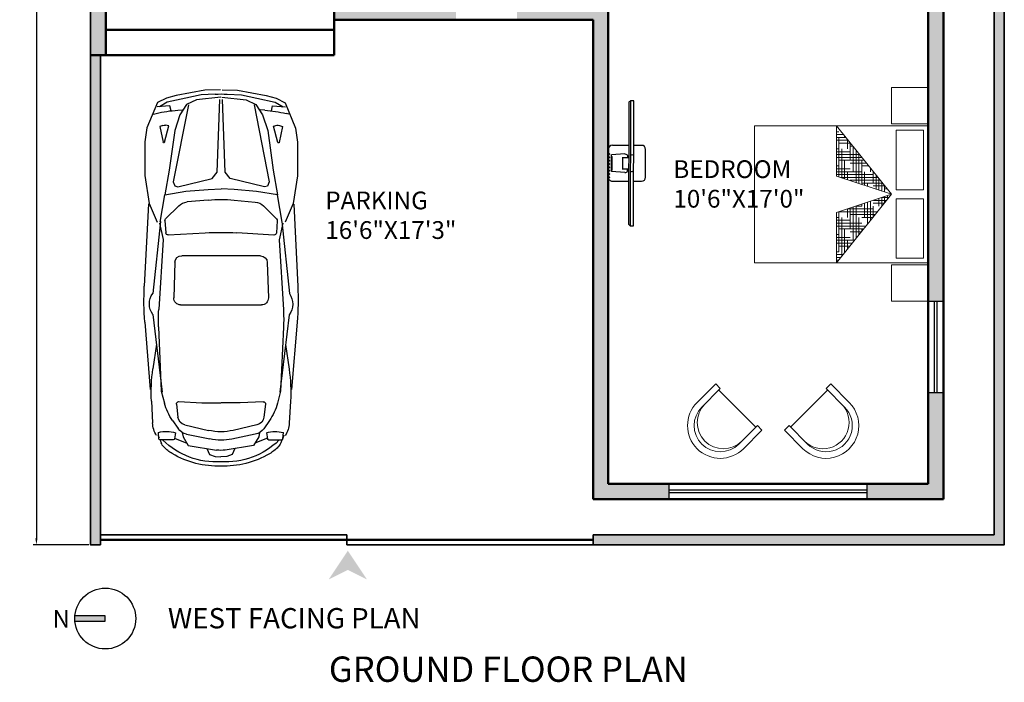
# Model space of a CAD drawing. Units: inches. Extents: x 2638 to 4577, y 1946 to 2619.
# Tile 1 of 8: x 2638 to 3025, y 1946 to 2207. Entities that reach past the tile are written whole.
import ezdxf

# ---------------------------------------------------------------- set-up
doc = ezdxf.new("R2010")
doc.units = ezdxf.units.IN
for name, color, linetype, lineweight in [('A-ANNO-DIMS', 2, 'Continuous', 18), ('A-ANNO-SYMB', 1, 'Continuous', 25), ('A-ANNO-TEXT', 7, 'Continuous', 25), ('A-AREA-IDEN', 7, 'Continuous', 25), ('A-FURN', 8, 'Continuous', 18), ('A-GLAZ', 4, 'Continuous', 25), ('A-WALL', 7, 'Continuous', 50), ('A-WALL-PATT', 8, 'Continuous', 13), ('C-PROP', 1, 'Continuous', 35), ('C-PROP-PATT', 252, 'Continuous', 13)]:
    doc.layers.add(name, color=color, linetype=linetype, lineweight=lineweight)
doc.layers.add('L9012X$0', color=2, linetype='Continuous')
doc.layers.add('window', color=130, linetype='Continuous')
doc.styles.get("Standard").update_dxf_attribs({"font": 'arial.ttf'})
doc.dimstyles.new('ISO-25', dxfattribs={"dimtxt": 5, "dimasz": 2.5, "dimexe": 1.25, "dimexo": 0.625, "dimtad": 1, "dimdec": 1, "dimlunit": 3, "dimtxsty": 'Standard', "dimcen": 2.5, "dimclrt": 1, "dimadec": 0, "dimazin": 0, "dimtfac": 1, "dimtdec": 1, "dimtmove": 0, "dimatfit": 3, "dimfxl": 1, "dimarcsym": 0})

# ---------------------------------------------------------------- blocks, each defined once
blk = doc.blocks.new('*D2')
at = {"layer": 'A-ANNO-DIMS', "color": 0, "lineweight": -2, "transparency": 16777216}
for p, q in [((2664.78, 2600.16), (2642.86, 2600.16)), ((2644.11, 2597.66), (2644.11, 2002.66)), ((2664.78, 2000.16), (2642.86, 2000.16))]:
    blk.add_line(p, q, dxfattribs=at)
at = {"layer": 'A-ANNO-DIMS', "color": 0, "transparency": 16777216}
for points in [[(2643.7, 2597.66), (2644.53, 2597.66), (2644.11, 2600.16)], [(2643.7, 2002.66), (2644.53, 2002.66), (2644.11, 2000.16)]]:
    blk.add_solid(points, dxfattribs=at)
at = {"layer": 'Defpoints', "color": 0, "transparency": 16777216}
for p in [(2665.41, 2600.16), (2644.11, 2000.16), (2665.41, 2000.16)]:
    blk.add_point(p, dxfattribs=at)
at = {"layer": 'A-ANNO-DIMS', "color": 0, "transparency": 16777216, "insert": (2640.93, 2300.16), "char_height": 5, "attachment_point": 5, "rotation": 90}
blk.add_mtext("50'", dxfattribs=at)
blk = doc.blocks.new('*X22')
at = {"color": 0}
for p, q in [((20.174, 14.75), (20.277, 14.75)), ((20.188, 14.75), (20.188, 14.767)), ((20.199, 14.781), (20.277, 14.781)), ((20.25, 14.812), (20.277, 14.812)), ((20.25, 14.319), (20.25, 14.75)), ((20.094, 14.375), (20.094, 14.65)), ((20.098, 14.656), (20.125, 14.656)), ((20.124, 14.688), (20.25, 14.688)), ((20.125, 14.5), (20.125, 14.689)), ((20.149, 14.719), (20.277, 14.719)), ((20.156, 14.625), (20.156, 14.728)), ((19.998, 14.531), (20.277, 14.531)), ((20.023, 14.562), (20.277, 14.562)), ((20.031, 14.247), (20.031, 14.573)), ((20.062, 14.257), (20.062, 14.612)), ((20.125, 14.594), (20.277, 14.594)), ((20.219, 14.309), (20.219, 14.625)), ((20.25, 14.625), (20.277, 14.625)), ((19.922, 14.438), (20, 14.438)), ((19.948, 14.469), (20.125, 14.469)), ((19.973, 14.5), (20.25, 14.5)), ((20, 14.237), (20, 14.5)), ((20.188, 14.299), (20.188, 14.5)), ((20.25, 14.438), (20.277, 14.438)), ((19.844, 14.185), (19.844, 14.34)), ((19.875, 14.25), (19.875, 14.379)), ((19.875, 14.344), (20.277, 14.344)), ((19.906, 14.375), (19.906, 14.417)), ((19.969, 14.226), (19.969, 14.375)), ((20, 14.375), (20.277, 14.375)), ((20.125, 14.406), (20.277, 14.406)), ((20.156, 14.288), (20.156, 14.375)), ((19.746, 14.219), (19.875, 14.219)), ((19.75, 14.154), (19.75, 14.223)), ((19.772, 14.25), (20, 14.25)), ((19.781, 14.164), (19.781, 14.262)), ((19.797, 14.281), (20.125, 14.281)), ((19.812, 14.174), (19.812, 14.301)), ((19.822, 14.312), (20.229, 14.312)), ((19.938, 14.216), (19.938, 14.25)), ((19.719, 14.073), (19.719, 14.114)), ((19.721, 14.188), (19.75, 14.188)), ((19.75, 14.034), (19.75, 14.103)), ((19.702, 14.094), (19.779, 14.094)), ((19.727, 14.062), (19.873, 14.062)), ((19.752, 14.031), (19.875, 14.031)), ((19.781, 13.995), (19.781, 14.093)), ((19.812, 14), (19.812, 14.082)), ((19.875, 13.878), (19.875, 14)), ((19.906, 13.84), (19.906, 14.051)), ((19.938, 13.801), (19.938, 14.041)), ((19.969, 13.875), (19.969, 14.031)), ((20, 14), (20, 14.02)), ((20, 14), (20.061, 14)), ((20.062, 13.645), (20.062, 14)), ((19.827, 13.938), (20.25, 13.938)), ((19.853, 13.906), (20.125, 13.906)), ((19.875, 13.969), (20.156, 13.969)), ((20.094, 13.625), (20.094, 13.989)), ((20.125, 13.75), (20.125, 13.979)), ((20.156, 13.875), (20.156, 13.969)), ((20.25, 13.5), (20.25, 13.937)), ((19.878, 13.875), (20, 13.875)), ((19.953, 13.781), (20.277, 13.781)), ((20, 13.812), (20.277, 13.812)), ((20.031, 13.684), (20.031, 13.875)), ((20.125, 13.844), (20.277, 13.844)), ((20.219, 13.451), (20.219, 13.875)), ((20.25, 13.875), (20.277, 13.875)), ((19.978, 13.75), (20.25, 13.75)), ((20, 13.723), (20, 13.75)), ((20.003, 13.719), (20.125, 13.719)), ((20.188, 13.49), (20.188, 13.75)), ((20.25, 13.688), (20.277, 13.688)), ((20.079, 13.625), (20.277, 13.625)), ((20.104, 13.594), (20.277, 13.594)), ((20.125, 13.656), (20.277, 13.656)), ((20.129, 13.562), (20.25, 13.562)), ((20.156, 13.529), (20.156, 13.625)), ((20.205, 13.469), (20.277, 13.469)), ((20.25, 13.5), (20.277, 13.5)), ((20.23, 13.438), (20.277, 13.438)), ((20.255, 13.406), (20.277, 13.406))]:
    blk.add_line(p, q, dxfattribs=at)
blk = doc.blocks.new('MAT-P02')
for p, q in [((-1.17, 0), (-1.17, -0.4)), ((-1.17, 0), (-0.77, 0)), ((-0.77, 0), (-0.77, -0.4)), ((-0.75, 0), (0.75, 0)), ((-0.75, 0), (-0.75, -1.9)), ((0.75, 0), (0.75, -1.9)), ((0.77, 0), (1.17, 0)), ((0.77, 0), (0.77, -0.4)), ((1.17, 0), (1.17, -0.4)), ((-0.7, -0.05), (-0.7, -0.35)), ((-0.7, -0.05), (-0.05, -0.05)), ((-0.05, -0.35), (-0.05, -0.05)), ((0.05, -0.05), (0.7, -0.05)), ((0.05, -0.35), (0.05, -0.05)), ((0.7, -0.05), (0.7, -0.35)), ((-1.17, -0.4), (-0.77, -0.4)), ((-0.75, -1.003), (0, -0.4)), ((0, -0.4), (-0.75, -1.003)), ((-0.7, -0.35), (-0.05, -0.35)), ((0, -0.4), (-0.2, -1.003)), ((0, -0.4), (0.2, -1.003)), ((0, -0.4), (0.75, -1.003)), ((0.05, -0.35), (0.7, -0.35)), ((0.77, -0.4), (1.17, -0.4)), ((-0.75, -1.003), (-0.2, -1.003)), ((0.2, -1.003), (0.75, -1.003)), ((0.75, -1.9), (-0.75, -1.9))]:
    blk.add_line(p, q)
at = {"xscale": -1, "rotation": 90}
blk.add_blockref('*X22', (14.128, 19.274), dxfattribs=at)
blk = doc.blocks.new('12PSTG07')
at = {"color": 0, "linetype": 'ByBlock'}
for p, q in [((0, 15), (-12, 15)), ((0, 12), (0, 15)), ((-12, 12), (0, 12)), ((-1, -12), (-1, 12)), ((-12, -12), (0, -12)), ((0, -12), (0, -15)), ((0, -15), (-12, -15))]:
    blk.add_line(p, q, dxfattribs=at)
for centre, radius in [((-12, 0), 15), ((-12, 0), 12), ((-10, 0), 12)]:
    blk.add_arc(centre, radius, 90, 270, dxfattribs=at)
blk = doc.blocks.new('A1099DC')
at = {"color": 0, "linetype": 'ByBlock'}
for p, q in [((1279.298465, 804.448389), (2201.430588, 851.890505)), ((2602.736326, 846.078152), (3356.693814, 785.353187)), ((3488.458929, 772.663345), (3732.658862, 759.86454)), ((139.051458, 595.027331), (190.951238, 683.213377)), ((179.200345, 564.515703), (190.951238, 709.631982)), ((272.228253, 749.073842), (265.114727, 718.465169)), ((398.733388, 644.315148), (411.280494, 678.748261)), ((411.280494, 678.748261), (588.616917, 641.417897)), ((1482.852352, 674.283145), (1175.286956, 622.180789)), ((1475.52921, 670.226262), (2282.402739, 758.004075)), ((1494.603245, 682.841284), (1678.210958, 641.166865)), ((1678.210958, 641.166865), (2462.684993, 690.847736)), ((2519.280414, 756.817792), (3387.476361, 653.818028)), ((2656.476214, 692.831247), (3376.704709, 662.004075)), ((2851.341839, 715.213377), (3126.60716, 755.701993)), ((3376.704709, 662.004075), (3510.708679, 626.736433)), ((3909.27561, 688.812956), (3837.725727, 693.401722)), ((3867.794139, 700.329656), (3900.059395, 686.767505)), ((3921.162781, 527.618662), (3921.162781, 676.138994)), ((3925.383812, 676.122818), (3955.306409, 663.545364)), ((92.537504, 388.14361), (139.051458, 595.027331)), ((236.043912, 551.980927), (179.200345, 564.515703)), ((405.405047, 577.538958), (396.874865, 615.894428)), ((589.014326, 626.599587), (405.405047, 577.538958)), ((1300.814287, 466.658131), (1445.712032, 613.104998)), ((1465.665584, 620.56924), (1602.893878, 610.287296)), ((1626.354615, 583.507504), (1602.652901, 169.222264)), ((229.117398, 477.634662), (225.714299, 427.957563)), ((1933.148906, 509.557888), (2330.980062, 522.200075)), ((2409.60024, 445.938054), (2410.49349, -460.09121)), ((3493.960271, 465.734554), (3507.923021, 209.166865)), ((3522.252709, 492.345257), (3666.066199, 475.644444)), ((3704.596898, 536.993674), (3795.675135, 473.385795)), ((3841.786866, 503.451367), (3910.58243, 515.096797)), ((3901.001848, 514.780764), (3957.150905, 375.772812)), ((57.774444, 216.608726), (92.537504, 388.14361)), ((1235.045743, 136.116317), (1257.419842, 373.755108)), ((1860.238743, -448.635916), (1859.369151, 433.397797)), ((3753.293176, 397.789551), (3815.226005, 132.124765)), ((3839.396146, 426.841284), (3888.358202, 417.538958)), ((3857.610793, 379.525702), (3912.067615, 118.157673)), ((3888.358202, 417.538958), (3983.199613, 359.957848)), ((3983.199613, 359.957848), (4035.448301, 43.94997)), ((49.168662, 58.00681), (57.774444, 216.608726)), ((3507.923021, 209.166865), (3507.64153, -4.333678)), ((4019.086894, 150.376168), (4084.69605, 122.469191)), ((4084.69605, 122.469191), (4109.177079, 60.329656)), ((4109.177079, 60.329656), (4113.094043, -5.158716)), ((49.301278, -76.507426), (58.219773, -235.092064)), ((3508.347273, -221.154823), (3507.644805, -7.65525)), ((3983.920268, -371.008369), (4035.545755, -54.898082)), ((4084.948231, -133.320044), (4109.306686, -71.132359)), ((4109.306686, -71.132359), (4113.094514, -5.636391)), ((1235.330373, -152.586046), (1258.173002, -390.180259)), ((1627.520644, -599.204785), (1603.002095, -184.967086)), ((3754.088875, -409.293325), (3815.497749, -143.506937)), ((3858.370276, -390.823819), (3912.311631, -129.348921)), ((4019.394229, -161.356334), (4084.948231, -133.320044)), ((58.219773, -235.092064), (93.320996, -406.558069)), ((3494.890446, -477.749545), (3508.347273, -221.154823)), ((93.320996, -406.558069), (140.24279, -613.349673)), ((3840.248961, -438.175225), (3889.19258, -428.776374)), ((3889.19258, -428.776374), (3983.920268, -371.008369)), ((3902.027941, -525.993061), (3957.902795, -386.874665)), ((230.077082, -495.779641), (226.576036, -446.109349)), ((1301.750547, -482.997536), (1446.936772, -629.158411)), ((1934.168526, -524.650381), (2332.023837, -536.508105)), ((3523.2353, -504.304409), (3667.01558, -487.320059)), ((3705.667171, -548.593196), (3796.61981, -484.805853)), ((3842.790735, -514.780444), (3911.609128, -526.290202)), ((3922.214148, -538.79118), (3922.506998, -687.311224)), ((140.24279, -613.349673), (192.316354, -701.433212)), ((237.150178, -570.112104), (180.331436, -582.758939)), ((180.331436, -582.758939), (192.368445, -727.851766)), ((406.561378, -595.336142), (398.106841, -633.708356)), ((590.267037, -644.034637), (406.561378, -595.336142)), ((412.636377, -696.533662), (589.898847, -658.853701)), ((1484.19765, -690.263206), (1176.530118, -638.767405)), ((1466.905004, -636.583294), (1604.112757, -626.030785)), ((1495.965396, -698.798158), (1679.490579, -656.761786)), ((1679.490579, -656.761786), (2464.061049, -704.895745)), ((3378.022114, -674.249887), (3511.956283, -638.718087)), ((273.723073, -767.133288), (266.549207, -736.538701)), ((400.0214, -662.125356), (412.636377, -696.533662)), ((1476.866524, -686.22077), (2283.911563, -772.40743)), ((2520.786439, -770.754078), (3388.777604, -666.042617)), ((2657.855804, -706.497136), (3378.022114, -674.249887)), ((2852.765183, -728.494989), (3128.109803, -768.440762)), ((3489.994314, -784.688586), (3734.168535, -771.408296)), ((3910.644841, -700.0086), (3839.104145, -704.738438)), ((3869.186159, -711.60707), (3901.424611, -697.981326)), ((3926.727989, -687.286725), (3956.625729, -674.650294)), ((1280.900818, -820.829563), (2203.124693, -866.453338)), ((2604.418191, -859.849707), (3358.254477, -797.638217))]:
    blk.add_line(p, q, dxfattribs=at)
for points in [[(-0.000783, 0.794772), (5.385043, 172.701749), (63.649891, 493.818028), (92.537504, 603.957563), (144.437284, 705.166865), (428.417214, 824.236633), (585.095796, 846.190121), (961.406447, 846.190121), (1274.27399, 797.818028), (1482.852352, 709.631982)], [(83.345007, -3.206171), (111.32237, 268.957533), (164.563706, 379.583828), (279.999271, 453.709838), (456.549665, 511.628518), (901.254996, 574.918954), (1175.286956, 622.180789), (1137.52997, 385.548359), (1118.345181, 137.317882), (1109.829198, -8.358455)], [(168.178729, 359.003083), (1030.214866, 528.397865), (1077.798844, 510.531569), (1086.170082, 475.285426), (992.832238, 91.960378), (924.218938, 35.478085), (108.447994, 6.034416)], [(0.019119, -19.392451), (5.743899, -191.288474), (64.641806, -512.289243), (93.746535, -622.371603), (145.845778, -723.478374), (430.059935, -841.987962), (586.7815, -863.632471), (963.091723, -863.198028), (1275.863278, -814.209121), (1484.26735, -725.611974)], [(83.356858, -15.227176), (111.870816, -287.335185), (165.330179, -397.856284), (280.911681, -471.754535), (457.575935, -529.324983), (902.4055, -592.045995), (1176.530118, -638.767405), (1138.306616, -402.209884), (1118.632407, -154.017717), (1109.829198, -8.358455)], [(168.904615, -377.268451), (1031.273389, -545.270714), (1078.822046, -527.310627), (1087.123771, -492.048047), (993.030273, -108.907787), (924.305735, -52.560894), (108.478017, -24.418246)]]:
    blk.add_lwpolyline(points, dxfattribs=at)
for centre, radius, start, end in [((2358.037832, -2192.08357), 3048, 85.395244, 92.945173), ((2399.99649, 588.663508), 206.166238, 54.649181, 124.776949), ((3392.740754, -1053.630025), 1828.8, 86.999806, 98.367602), ((1749.553982, 373.478072), 1524, 166.916578, 176.08111), ((2578.271641, -1134.295865), 1828.8, 87.549126, 93.623712), ((3718.678317, 475.802507), 284.405862, 57.329946, 87.182375), ((4191.049821, 605.937201), 363.988953, 166.096081, 196.353514), ((3908.462781, 676.138994), 12.7, 0, 86.330429), ((3896.252417, 523.051998), 152.4, 46.38363, 67.20138), ((446.46332, 626.922805), 50.8, 159.97873, 192.538409), ((587.047263, 633.961317), 7.62, 284.960009, 78.112462), ((1463.767788, 595.240237), 25.4, 85.715073, 135.304647), ((1600.996082, 584.958293), 25.4, 356.725615, 85.715073), ((3355.555414, 37.211519), 609.6, 55.070043, 75.255062), ((3320.85101, 50.338397), 847.430844, 356.245089, 44.519453), ((3700.933354, 318.064082), 435.542335, 30.457681, 46.38363), ((1409.148822, 359.469565), 152.4, 135.304647, 174.62136), ((1935.569151, 433.396333), 76.2, 91.82012, 179.9989), ((2333.400307, 446.03852), 76.2, 359.924458, 91.82012), ((3519.322741, 467.114813), 25.4, 83.37601, 183.115039), ((3654.346327, 374.722669), 101.6, 13.122645, 83.37601), ((3708.414764, 348.440256), 152.4, 11.769371, 55.070043), ((3908.462781, 527.618662), 12.7, 279.607718, 0), ((3204.184594, 25.950693), 1011.814461, 358.069446, 30.457681), ((2752.335538, -6.739118), 1524, 174.62136, 185.491615), ((4645.676894, -4.872483), 3048, 176.725615, 183.38736), ((3221.54491, -6.276527), 609.6, 346.99033, 13.122645), ((3315.283499, -6.18411), 609.6, 348.343604, 11.769371), ((1266.577845, -8.050136), 1219.2, 176.894161, 183.218814), ((3734.73098, -5.770579), 304.8, 350.724636, 9.388339), ((3320.962449, -62.69553), 847.430844, 315.593523, 3.867886), ((3204.248172, -38.537915), 1011.814461, 329.655294, 2.043529), ((1409.873518, -375.595566), 152.4, 185.491615, 224.808328), ((3655.096735, -386.42159), 101.6, 276.736965, 346.99033), ((3709.113243, -360.032616), 152.4, 305.042932, 348.343604), ((1750.305335, -388.625277), 1524, 184.031865, 193.196397), ((1936.438592, -448.484202), 76.2, 180.114076, 268.292856), ((2334.293902, -460.341926), 76.2, 268.292856, 0.188517), ((3520.255588, -479.079792), 25.4, 176.997936, 276.736965), ((3355.640902, -49.500248), 609.6, 284.857913, 305.042932), ((4192.255091, -616.577407), 363.988953, 163.759461, 194.016894), ((3909.514173, -538.816222), 12.7, 0.112975, 80.505257), ((3701.571953, -329.671253), 435.542335, 313.729345, 329.655294), ((447.716945, -644.638934), 50.8, 167.574566, 200.134245), ((588.314493, -651.400231), 7.62, 282.000513, 75.152966), ((1464.957267, -611.258083), 25.4, 224.808328, 274.397903), ((1602.165021, -600.705574), 25.4, 274.397903, 3.38736), ((3897.294828, -534.273643), 152.4, 292.911596, 313.729345), ((2401.171182, -602.835323), 206.166238, 235.336026, 305.463794), ((2576.048678, 1120.472221), 1828.8, 266.489263, 272.563849), ((3390.675263, 1041.412497), 1828.8, 261.745373, 273.113169), ((3719.627907, -487.374382), 284.405862, 272.930601, 302.78303), ((3909.807023, -687.336265), 12.7, 273.782546, 0.112975), ((2353.729565, 2177.823616), 3048, 267.167802, 274.717731)]:
    blk.add_arc(centre, radius, start, end, dxfattribs=at)
blk = doc.blocks.new('VI')
at = {"layer": 'L9012X$0'}
blk.add_blockref('A1099DC', (0, 0), dxfattribs=at)
blk = doc.blocks.new('TV')
at = {"color": 0}
for p, q in [((3967.27, 1784.85), (3967.05, 1784.65)), ((3967.76, 1763.68), (3967.54, 1763.86))]:
    blk.add_line(p, q, dxfattribs=at)
at = {"layer": 'window'}
for p, q in [((3967.54, 1763.86), (3967.05, 1784.65)), ((3964.41, 1777.23), (3967.22, 1777.3)), ((3968.01, 1777.32), (3969.36, 1777.35)), ((3966.53, 1775.82), (3964.33, 1775.61)), ((3964.34, 1775.34), (3964.45, 1775.34)), ((3964.34, 1775.31), (3964.43, 1775.32)), ((3966.14, 1775.2), (3967.01, 1775.22)), ((3966.14, 1775.18), (3967.27, 1775.2)), ((3966.14, 1775.18), (3966.14, 1775.2)), ((3966.3, 1773.29), (3966.26, 1775.18)), ((3966.19, 1773.28), (3967.31, 1773.31)), ((3964.39, 1773.06), (3964.48, 1773.06)), ((3964.39, 1773.04), (3964.5, 1773.04)), ((3966.61, 1772.66), (3964.4, 1772.77)), ((3966.19, 1773.26), (3967.05, 1773.28)), ((3966.19, 1773.26), (3966.19, 1773.28)), ((3964.55, 1771.15), (3967.36, 1771.22)), ((3968.15, 1771.24), (3969.5, 1771.27))]:
    blk.add_line(p, q, dxfattribs=at)
for points in [[(3968.33, 1763.69), (3967.83, 1784.86), (3967.27, 1784.85), (3967.76, 1763.68), (3968.33, 1763.69)], [(3970.16, 1771.96), (3970.05, 1776.69)], [(3963.86, 1771.81), (3963.75, 1776.54)], [(3964.4, 1772.77), (3964.33, 1775.61)], [(3964.48, 1773.06), (3964.43, 1775.32)], [(3964.5, 1773.04), (3964.45, 1775.34)]]:
    blk.add_lwpolyline(points, dxfattribs=at)
for points in [[(3966.53, 1775.82, -0.263666), (3966.93, 1775.69), (3967, 1775.57), (3967.01, 1775.22)], [(3966.61, 1772.66, 0.263666), (3967, 1772.81), (3967.06, 1772.93), (3967.05, 1773.28)]]:
    blk.add_lwpolyline(points, format="xyb", dxfattribs=at)
for centre, radius in [((3963.91, 1775.73), 0.0679), ((3963.93, 1775.17), 0.0679), ((3967.77, 1775.68), 0.0451), ((3963.94, 1774.6), 0.0679), ((3963.95, 1774.04), 0.0679), ((3963.97, 1773.48), 0.0679), ((3963.98, 1772.92), 0.0679), ((3963.99, 1772.35), 0.0679), ((3964.01, 1771.79), 0.0679), ((3967.83, 1772.86), 0.0451)]:
    blk.add_circle(centre, radius, dxfattribs=at)
for centre, start, end in [((3964.42, 1776.56), 91.3414, 181.3414), ((3969.38, 1776.67), 1.3414, 91.3414), ((3964.53, 1771.83), 181.3414, 271.3414), ((3969.49, 1771.94), 271.3414, 1.3414)]:
    blk.add_arc(centre, 0.676, start, end, dxfattribs=at)
blk = doc.blocks.new('WIN-36')
for p, q in [((2761.41, 2540.16), (2761.41, 2534.16)), ((2761.41, 2537.66), (2797.41, 2537.66)), ((2797.41, 2540.16), (2797.41, 2534.16)), ((2761.41, 2536.66), (2797.41, 2536.66))]:
    blk.add_line(p, q)
blk = doc.blocks.new('WIN-78')
for p, q in [((3314.99, 2024.16), (3314.99, 2018.16)), ((3314.99, 2021.66), (3392.99, 2021.66)), ((3392.99, 2024.16), (3392.99, 2018.16)), ((3314.99, 2020.66), (3392.99, 2020.66))]:
    blk.add_line(p, q)

msp = doc.modelspace()

# ---------------------------------------------------------------- hatches: boundary and pattern name
at = {"layer": 'A-ANNO-SYMB', "transparency": 33554687}
h = msp.add_hatch(color=256, dxfattribs=at)
h.dxf.hatch_style = 1
h.paths.add_polyline_path([(2766.79, 1990.28), (2774.34, 1986.51), (2766.79, 1997.83), (2759.24, 1986.51)])
h = msp.add_hatch(color=256, dxfattribs=at)
h.dxf.hatch_style = 1
h.paths.add_polyline_path([(2671.23, 1972.11), (2671.23, 1970.11), (2659.27, 1970.11, -0.020861), (2659.23, 1971.11, -0.020861), (2659.27, 1972.11)])
at = {"layer": 'A-WALL-PATT', "transparency": 33554687}
h = msp.add_hatch(color=256, dxfattribs=at)
h.dxf.hatch_style = 1
h.paths.add_polyline_path([(2749.41, 2558.16), (2689.41, 2558.16), (2689.41, 2472.16), (2695.41, 2472.16), (2695.41, 2476.16), (2701.41, 2476.16), (2701.41, 2480.16), (2695.41, 2480.16), (2695.41, 2552.16), (2743.41, 2552.16), (2743.41, 2480.16), (2737.41, 2480.16), (2737.41, 2476.16), (2747.41, 2476.16), (2747.41, 2534.16), (2761.41, 2534.16), (2761.41, 2540.16), (2749.41, 2540.16)])
h.paths.add_polyline_path([(2803.41, 2540.16), (2797.41, 2540.16), (2797.41, 2534.16), (2803.41, 2534.16)])
h.paths.add_polyline_path([(2905.41, 2558.16), (2857.41, 2558.16), (2857.41, 2540.16), (2839.44, 2540.16), (2839.44, 2540.16), (2839.41, 2534.26), (2839.41, 2534.16), (2859.41, 2534.16), (2859.41, 2516.16), (2863.41, 2516.16), (2863.41, 2552.16), (2905.41, 2552.16)])
h.paths.add_polyline_path([(3001.41, 2558.16), (2929.41, 2558.16), (2929.41, 2552.16), (2995.41, 2552.16), (2995.41, 2522.16), (3001.41, 2522.16)])
h.paths.add_polyline_path([(3001.41, 2486.16), (2995.41, 2486.16), (2995.41, 2426.16), (2881.41, 2426.16), (2881.41, 2422.16), (2995.41, 2422.16), (2995.41, 2418.91), (3001.41, 2418.91)])
h.paths.add_polyline_path([(3001.41, 2382.91), (2995.41, 2382.91), (2995.41, 2336.41), (3001.41, 2336.41)])
h.paths.add_polyline_path([(3001.41, 2300.41), (2995.41, 2300.41), (2995.41, 2296.16), (2908.41, 2296.16), (2908.41, 2292.16), (2913.41, 2292.16), (2913.41, 2264.16), (2917.41, 2264.16), (2917.41, 2292.16), (2995.41, 2292.16), (2995.41, 2274.16), (3001.41, 2274.16)])
h.paths.add_polyline_path([(3001.41, 2250.16), (2995.41, 2250.16), (2995.41, 2232.16), (2917.41, 2232.16), (2917.41, 2234.16), (2913.41, 2234.16), (2913.41, 2228.16), (2995.41, 2228.16), (2995.41, 2096.16), (3001.41, 2096.16)])
h.paths.add_polyline_path([(3001.41, 2060.16), (2995.41, 2060.16), (2995.41, 2024.16), (2971.41, 2024.16), (2971.41, 2018.16), (3001.41, 2018.16)])
h.paths.add_polyline_path([(2869.41, 2292.16), (2872.41, 2292.16), (2872.41, 2296.16), (2863.41, 2296.16), (2863.41, 2213.16), (2833.41, 2213.16), (2833.41, 2207.16), (2863.41, 2207.16), (2863.41, 2018.16), (2893.41, 2018.16), (2893.41, 2024.16), (2869.41, 2024.16)])
h.paths.add_polyline_path([(2809.41, 2213.16), (2767.41, 2213.16), (2767.41, 2216.16), (2761.41, 2216.16), (2761.41, 2207.16), (2809.41, 2207.16)])
h.paths.add_polyline_path([(2671.41, 2290.16), (2761.41, 2290.16), (2761.41, 2288.16), (2767.41, 2288.16), (2767.41, 2290.16), (2791.41, 2290.16), (2791.41, 2296.16), (2695.41, 2296.16), (2695.41, 2320.16), (2689.41, 2320.16), (2689.41, 2296.16), (2665.41, 2296.16), (2665.41, 2193.16), (2671.41, 2193.16)])
h.paths.add_polyline_path([(2695.41, 2448.16), (2689.41, 2448.16), (2689.41, 2404.16), (2695.41, 2404.16)])
at = {"layer": 'C-PROP-PATT', "transparency": 33554687}
h = msp.add_hatch(color=256, dxfattribs=at)
h.dxf.hatch_style = 1
h.paths.add_polyline_path([(3025.41, 2600.16), (2665.41, 2600.16), (2665.41, 2296.16), (2669.41, 2296.16), (2669.41, 2596.16), (3021.41, 2596.16), (3021.41, 2004.16), (2863.41, 2004.16), (2863.41, 2000.16), (3025.41, 2000.16)])
h.paths.add_polyline_path([(2669.41, 2193.16), (2665.41, 2193.16), (2665.41, 2000.16), (2669.41, 2000.16)], flags=17)

# ---------------------------------------------------------------- linework, layer by layer
at = {"layer": 'A-ANNO-SYMB'}
for p, q in [((2671.23, 1972.11), (2659.27, 1972.11)), ((2671.23, 1970.11), (2671.23, 1972.11)), ((2659.23, 1970.11), (2671.23, 1970.11))]:
    msp.add_line(p, q, dxfattribs=at)
msp.add_circle((2671.23, 1971.11), 12, dxfattribs=at)
at = {"layer": 'A-WALL'}
for p, q in [((3001.41, 2558.16), (3001.41, 2018.16)), ((2671.41, 2193.16), (2671.41, 2290.16)), ((2869.41, 2292.16), (2869.41, 2024.16)), ((2995.41, 2228.16), (2995.41, 2024.16)), ((2761.41, 2216.16), (2761.41, 2193.16)), ((2863.41, 2207.16), (2761.41, 2207.16)), ((2863.41, 2207.16), (2863.41, 2018.16)), ((2761.41, 2203.16), (2671.41, 2203.16)), ((2761.41, 2193.16), (2665.41, 2193.16)), ((2995.41, 2024.16), (2869.41, 2024.16)), ((3001.41, 2018.16), (2863.41, 2018.16)), ((2863.41, 2002.16), (2669.41, 2002.16))]:
    msp.add_line(p, q, dxfattribs=at)
at = {"layer": 'C-PROP'}
for p, q in [((2669.41, 2004.16), (2766.41, 2004.16)), ((2766.41, 2002.16), (2766.41, 2004.16)), ((2766.41, 2002.16), (2766.41, 2000.16)), ((2863.41, 2004.16), (2863.41, 2000.16)), ((2863.41, 2000.16), (2766.41, 2000.16))]:
    msp.add_line(p, q, dxfattribs=at)
for points in [[(2669.41, 2000.16), (2665.41, 2000.16), (2665.41, 2600.16), (3025.41, 2600.16), (3025.41, 2000.16), (2863.41, 2000.16)], [(2669.41, 2296.16), (2669.41, 2596.16), (3021.41, 2596.16), (3021.41, 2004.16), (2863.41, 2004.16)], [(2669.41, 2000.16), (2669.41, 2193.16)]]:
    msp.add_lwpolyline(points, dxfattribs=at)

# ---------------------------------------------------------------- block references
at = {"layer": 'A-FURN'}
for name, p, xscale, yscale, zscale, rotation in [('MAT-P02', (2995.41, 2138.32), 36.03633950593442, 36.03633950593442, 36.03633950593442, 270), ('VI', (2716.6, 2179.54), -0.0351896714874634, 0.0351896714874634, 0.0351896714874634, 90), ('TV', (-6457.62, -1742.61), 2.327319231123021, 2.327319231123021, 2.327319231123021, 358.5430845181613), ('12PSTG07', (2920.83, 2054.44), -0.8597921787217943, 0.8597921787217943, 0.8597921787217943, 225), ('12PSTG07', (2947.89, 2054.44), 0.8597921787217943, 0.8597921787217943, 0.8597921787217943, 134.9999999999999)]:
    msp.add_blockref(name, p, dxfattribs=dict(at, xscale=xscale, yscale=yscale, zscale=zscale, rotation=rotation))
at = {"layer": 'A-GLAZ'}
for name, p, rotation in [('WIN-36', (5535.57, -701.25), 90.00000000000281), ('WIN-78', (6286.4, 4042.31), 180)]:
    msp.add_blockref(name, p, dxfattribs=dict(at, rotation=rotation))

# ---------------------------------------------------------------- texts
at = {"layer": 'A-ANNO-SYMB'}
msp.add_text('N', height=6.9, dxfattribs=at).set_placement((2650.49, 1967.57))
at = {"layer": 'A-ANNO-TEXT', "attachment_point": 1}
for s, insert, char_height in [('{\\fTimes New Roman|b0|i0|c0|p18;WEST FACING PLAN}', (2695.92, 1975.23), 8), ('{\\fTimes New Roman|b0|i0|c0|p18;GROUND FLOOR PLAN}', (2759.32, 1956.14), 10)]:
    msp.add_mtext_dynamic_manual_height_columns(s, width=196.2607, gutter_width=12.5, heights=[0], dxfattribs=dict(at, insert=insert, char_height=char_height))
at = {"layer": 'A-AREA-IDEN', "char_height": 7, "attachment_point": 1}
for s, insert in [('{\\fTimes New Roman|b0|i0|c0|p18;BEDROOM\\P10\'6"X17\'0"}', (2895.04, 2151.74)), ('{\\fTimes New Roman|b0|i0|c0|p18;PARKING\\P16\'6"X17\'3"}', (2757.93, 2139.41))]:
    msp.add_mtext_dynamic_manual_height_columns(s, width=61.0557, gutter_width=12.5, heights=[0], dxfattribs=dict(at, insert=insert))

# ---------------------------------------------------------------- dimensions: what is measured, and where the dimension line sits
at = {"layer": 'A-ANNO-DIMS'}
dim = msp.add_linear_dim(base=(2644.11, 2000.16), p1=(2665.41, 2600.16), p2=(2665.41, 2000.16), angle=90, dimstyle='ISO-25', override={"dimclrd": 0, "dimclre": 0, "dimclrt": 0}, dxfattribs=at)
dim.commit()
dim.dimension.update_dxf_attribs({"geometry": '*D2', "text_midpoint": (2640.93, 2300.16)})

doc.saveas('drawing.dxf')
